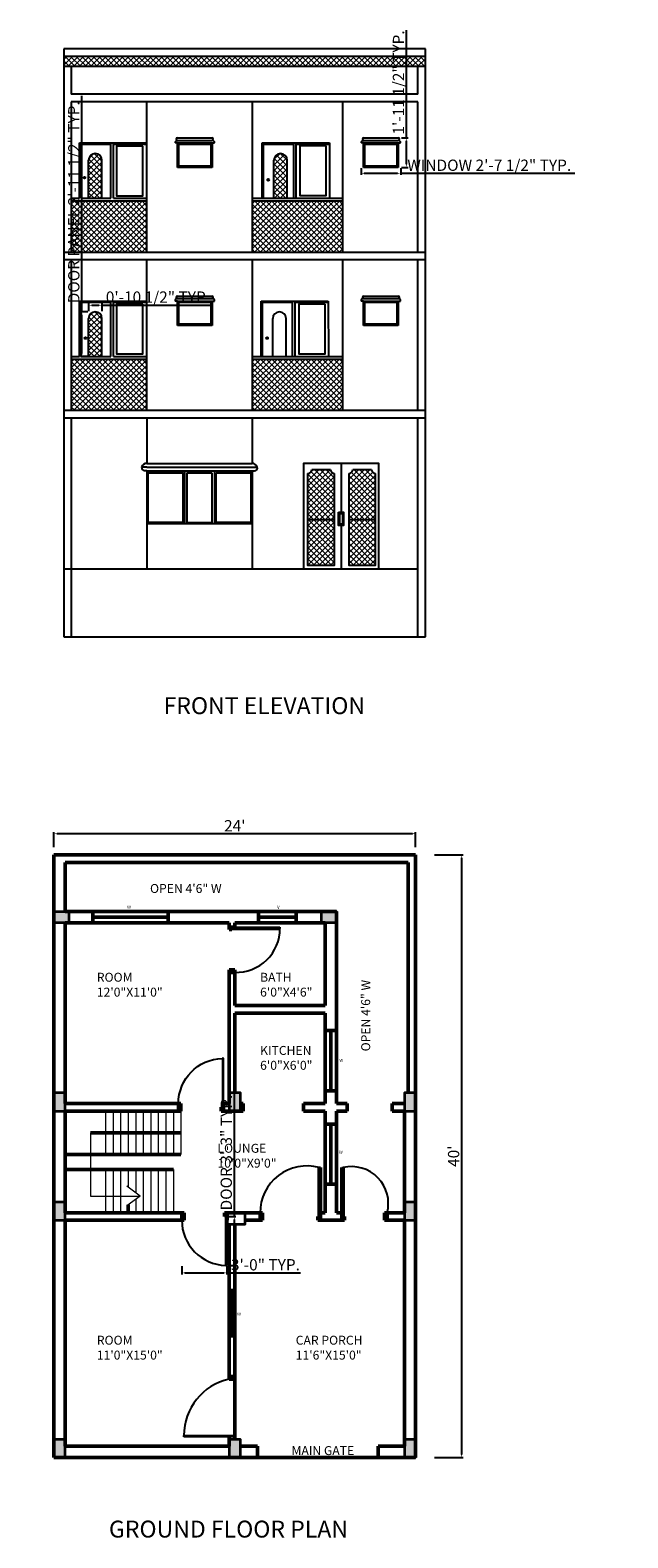
# Model space of a CAD drawing. Units: feet. Extents: x 1398 to 2768, y 682 to 1909.
# Tile 1 of 3: x 1398 to 1874, y 682 to 1883. Entities that reach past the tile are written whole.
import ezdxf

# ---------------------------------------------------------------- set-up
doc = ezdxf.new("R2010")
doc.units = ezdxf.units.FT
for name, color, linetype, lineweight in [('A-ANNO-DIMS', 2, 'Continuous', 18), ('A-ANNO-TEXT', 7, 'Continuous', 18), ('A-AREA-IDEN', 3, 'Continuous', 18), ('A-COLS', 7, 'Continuous', 35), ('A-DOOR', 4, 'Continuous', 25), ('A-ELEV', 7, 'Continuous', 25), ('A-ELEV-PATT', 8, 'Continuous', 13), ('A-FLOR-STRS', 3, 'Continuous', 18), ('A-WALL', 7, 'Continuous', 50), ('A-WALL-PATT', 8, 'Continuous', 13)]:
    doc.layers.add(name, color=color, linetype=linetype, lineweight=lineweight)
doc.styles.get("Standard").update_dxf_attribs({"font": 'arial.ttf'})
doc.dimstyles.new('ISO-25', dxfattribs={"dimtxt": 9, "dimasz": 2.5, "dimexe": 1.25, "dimexo": 0.625, "dimtad": 1, "dimdec": 1, "dimlunit": 3, "dimtxsty": 'Standard', "dimcen": 2.5, "dimadec": 0, "dimazin": 0, "dimtfac": 1, "dimtdec": 1, "dimtmove": 0, "dimatfit": 3, "dimfxl": 1, "dimarcsym": 0})
pattern_1 = [(45, (-71.1406, 0), (-2.245064, 2.245064), []), (135, (-71.1406, 0), (-2.245064, -2.245064), [])]

# ---------------------------------------------------------------- blocks, each defined once
blk = doc.blocks.new('*D1')
at = {"layer": 'A-ANNO-DIMS', "color": 0, "lineweight": -2, "transparency": 16777216}
for p, q in [((1416.8, 1232.1), (1416.8, 1244.2)), ((1702.3, 1242.9), (1419.3, 1242.9)), ((1704.8, 1232.1), (1704.8, 1244.2))]:
    blk.add_line(p, q, dxfattribs=at)
at = {"layer": 'A-ANNO-DIMS', "color": 0, "transparency": 16777216}
for points in [[(1419.3, 1243.4), (1419.3, 1242.5), (1416.8, 1242.9)], [(1702.3, 1243.4), (1702.3, 1242.5), (1704.8, 1242.9)]]:
    blk.add_solid(points, dxfattribs=at)
at = {"layer": 'Defpoints', "color": 0, "transparency": 16777216}
for p in [(1416.8, 1242.9), (1416.8, 1231.4), (1704.8, 1231.4)]:
    blk.add_point(p, dxfattribs=at)
at = {"layer": 'A-ANNO-DIMS', "color": 0, "transparency": 16777216, "insert": (1560.8, 1248.1), "char_height": 9, "attachment_point": 5}
blk.add_mtext("24'", dxfattribs=at)
blk = doc.blocks.new('*D2')
at = {"layer": 'A-ANNO-DIMS', "color": 0, "lineweight": -2, "transparency": 16777216}
for p, q in [((1719.8, 1226.1), (1742.7, 1226.1)), ((1741.4, 1223.6), (1741.4, 748.6)), ((1719.8, 746.1), (1742.7, 746.1))]:
    blk.add_line(p, q, dxfattribs=at)
at = {"layer": 'A-ANNO-DIMS', "color": 0, "transparency": 16777216}
for points in [[(1741, 1223.6), (1741.8, 1223.6), (1741.4, 1226.1)], [(1741, 748.6), (1741.8, 748.6), (1741.4, 746.1)]]:
    blk.add_solid(points, dxfattribs=at)
at = {"layer": 'Defpoints', "color": 0, "transparency": 16777216}
for p in [(1719.2, 1226.1), (1719.2, 746.1), (1741.4, 746.1)]:
    blk.add_point(p, dxfattribs=at)
at = {"layer": 'A-ANNO-DIMS', "color": 0, "transparency": 16777216, "insert": (1736.2, 986.1), "char_height": 9, "attachment_point": 5, "rotation": 90}
blk.add_mtext("40'", dxfattribs=at)
blk = doc.blocks.new('DOOR-PLAN-900')
for p, q in [((1553.6, 938.1), (1552.6, 938.1)), ((1553.6, 899.1), (1553.6, 938.1)), ((1554.6, 935.1), (1554.6, 899.1)), ((1554.6, 899.1), (1553.6, 899.1))]:
    blk.add_line(p, q)
blk.add_arc((1554.6, 935.1), 36, 180, 268.3861)
blk = doc.blocks.new('ELEV-WINDOW')
for p, q in [((2, 19.5), (0, 19.5)), ((2, 23.5), (29.5, 23.5)), ((2, 21.5), (29.5, 21.5)), ((2, 19.5), (29.5, 19.5)), ((2, 0), (2, 19.5)), ((29.5, 19.5), (29.5, 0)), ((29.5, 19.5), (31.5, 19.5)), ((29.5, 0), (2, 0))]:
    blk.add_line(p, q)
for centre, radius, start, end in [((2, 19.5), 2, 90, 180), ((2, 22.5), 1, 90, 270), ((29.5, 22.5), 1, 270, 90), ((29.5, 19.5), 2, 0, 90)]:
    blk.add_arc(centre, radius, start, end)
blk = doc.blocks.new('ELEV-DOOR')
for p, q in [((0, 0), (0, 30.3)), ((10.6, 0), (10.6, 30.3))]:
    blk.add_line(p, q)
blk.add_arc((5.3, 30.3), 5.3, 0, 180)
blk = doc.blocks.new('*D29')
at = {"layer": 'A-ANNO-DIMS', "color": 0, "lineweight": -2, "transparency": 16777216}
for p, q in [((1560.5, 938.1), (1560.5, 1037.5)), ((1555.2, 938.1), (1561.7, 938.1)), ((1560.5, 901.6), (1560.5, 935.6)), ((1555.2, 899.1), (1561.7, 899.1))]:
    blk.add_line(p, q, dxfattribs=at)
at = {"layer": 'A-ANNO-DIMS', "color": 0, "transparency": 16777216}
for points in [[(1560.1, 935.6), (1560.9, 935.6), (1560.5, 938.1)], [(1560.1, 901.6), (1560.9, 901.6), (1560.5, 899.1)]]:
    blk.add_solid(points, dxfattribs=at)
at = {"layer": 'Defpoints', "color": 0, "transparency": 16777216}
for p in [(1554.6, 938.1), (1560.5, 938.1), (1554.6, 899.1)]:
    blk.add_point(p, dxfattribs=at)
at = {"layer": 'A-ANNO-DIMS', "color": 0, "transparency": 16777216, "insert": (1555.2, 989), "char_height": 9, "attachment_point": 5, "rotation": 90}
blk.add_mtext('DOOR 3\'-3" TYP.', dxfattribs=at)
blk = doc.blocks.new('*D30')
at = {"layer": 'A-ANNO-DIMS', "color": 0, "lineweight": -2, "transparency": 16777216}
for p, q in [((1518.6, 898.5), (1518.6, 892)), ((1521.1, 893.2), (1552.1, 893.2)), ((1554.6, 898.5), (1554.6, 892)), ((1554.6, 893.2), (1613.2, 893.2))]:
    blk.add_line(p, q, dxfattribs=at)
at = {"layer": 'A-ANNO-DIMS', "color": 0, "transparency": 16777216}
for points in [[(1521.1, 893.6), (1521.1, 892.8), (1518.6, 893.2)], [(1552.1, 893.6), (1552.1, 892.8), (1554.6, 893.2)]]:
    blk.add_solid(points, dxfattribs=at)
at = {"layer": 'Defpoints', "color": 0, "transparency": 16777216}
for p in [(1518.6, 899.1), (1554.6, 899.1), (1554.6, 893.2)]:
    blk.add_point(p, dxfattribs=at)
at = {"layer": 'A-ANNO-DIMS', "color": 0, "transparency": 16777216, "insert": (1585.2, 898.5), "char_height": 9, "attachment_point": 5}
blk.add_mtext('3\'-0" TYP.', dxfattribs=at)
blk = doc.blocks.new('*D31')
at = {"layer": 'A-ANNO-DIMS', "color": 0, "lineweight": -2, "transparency": 16777216}
for p, q in [((1661.4, 1773), (1661.4, 1767.6)), ((1663.9, 1768.9), (1690.4, 1768.9)), ((1692.9, 1773), (1692.9, 1767.6)), ((1692.9, 1768.9), (1831.5, 1768.9))]:
    blk.add_line(p, q, dxfattribs=at)
at = {"layer": 'A-ANNO-DIMS', "color": 0, "transparency": 16777216}
for points in [[(1663.9, 1769.3), (1663.9, 1768.5), (1661.4, 1768.9)], [(1690.4, 1769.3), (1690.4, 1768.5), (1692.9, 1768.9)]]:
    blk.add_solid(points, dxfattribs=at)
at = {"layer": 'Defpoints', "color": 0, "transparency": 16777216}
for p in [(1661.4, 1773.6), (1692.9, 1773.6), (1692.9, 1768.9)]:
    blk.add_point(p, dxfattribs=at)
at = {"layer": 'A-ANNO-DIMS', "color": 0, "transparency": 16777216, "insert": (1763.4, 1774.1), "char_height": 9, "attachment_point": 5}
blk.add_mtext('WINDOW 2\'-7 1/2" TYP.', dxfattribs=at)
blk = doc.blocks.new('*D32')
at = {"layer": 'A-ANNO-DIMS', "color": 0, "lineweight": -2, "transparency": 16777216}
for p, q in [((1697.6, 1797.1), (1697.6, 1882.9)), ((1693.5, 1797.1), (1698.9, 1797.1)), ((1697.6, 1776.1), (1697.6, 1794.6)), ((1693.5, 1773.6), (1698.9, 1773.6))]:
    blk.add_line(p, q, dxfattribs=at)
at = {"layer": 'A-ANNO-DIMS', "color": 0, "transparency": 16777216}
for points in [[(1697.2, 1794.6), (1698, 1794.6), (1697.6, 1797.1)], [(1697.2, 1776.1), (1698, 1776.1), (1697.6, 1773.6)]]:
    blk.add_solid(points, dxfattribs=at)
at = {"layer": 'Defpoints', "color": 0, "transparency": 16777216}
for p in [(1692.9, 1797.1), (1697.6, 1797.1), (1692.9, 1773.6)]:
    blk.add_point(p, dxfattribs=at)
at = {"layer": 'A-ANNO-DIMS', "color": 0, "transparency": 16777216, "insert": (1692.3, 1841.2), "char_height": 9, "attachment_point": 5, "rotation": 90}
blk.add_mtext('1\'-11 1/2" TYP.', dxfattribs=at)
blk = doc.blocks.new('*D33')
at = {"layer": 'A-ANNO-DIMS', "color": 0, "lineweight": -2, "transparency": 16777216}
for p, q in [((1439.1, 1658.5), (1439.1, 1830.6)), ((1443.8, 1658.5), (1437.9, 1658.5)), ((1439.1, 1625.4), (1439.1, 1656)), ((1443.8, 1622.9), (1437.9, 1622.9))]:
    blk.add_line(p, q, dxfattribs=at)
at = {"layer": 'A-ANNO-DIMS', "color": 0, "transparency": 16777216}
for points in [[(1438.7, 1656), (1439.5, 1656), (1439.1, 1658.5)], [(1438.7, 1625.4), (1439.5, 1625.4), (1439.1, 1622.9)]]:
    blk.add_solid(points, dxfattribs=at)
at = {"layer": 'Defpoints', "color": 0, "transparency": 16777216}
for p in [(1439.1, 1658.5), (1444.5, 1658.5), (1444.5, 1622.9)]:
    blk.add_point(p, dxfattribs=at)
at = {"layer": 'A-ANNO-DIMS', "color": 0, "transparency": 16777216, "insert": (1433.8, 1745.8), "char_height": 9, "attachment_point": 5, "rotation": 90}
blk.add_mtext('DOOR PANEL 2\'-11 1/2" TYP.', dxfattribs=at)
blk = doc.blocks.new('*D34')
at = {"layer": 'A-ANNO-DIMS', "color": 0, "lineweight": -2, "transparency": 16777216}
for p, q in [((1444.5, 1659.1), (1444.5, 1665.1)), ((1447, 1663.8), (1452.6, 1663.8)), ((1455.1, 1659.1), (1455.1, 1665.1)), ((1455.1, 1663.8), (1541.6, 1663.8))]:
    blk.add_line(p, q, dxfattribs=at)
at = {"layer": 'A-ANNO-DIMS', "color": 0, "transparency": 16777216}
for points in [[(1447, 1664.2), (1447, 1663.4), (1444.5, 1663.8)], [(1452.6, 1664.2), (1452.6, 1663.4), (1455.1, 1663.8)]]:
    blk.add_solid(points, dxfattribs=at)
at = {"layer": 'Defpoints', "color": 0, "transparency": 16777216}
for p in [(1444.5, 1658.5), (1455.1, 1663.8), (1455.1, 1658.5)]:
    blk.add_point(p, dxfattribs=at)
at = {"layer": 'A-ANNO-DIMS', "color": 0, "transparency": 16777216, "insert": (1499.6, 1669.1), "char_height": 9, "attachment_point": 5}
blk.add_mtext('0\'-10 1/2" TYP.', dxfattribs=at)

msp = doc.modelspace()

# ---------------------------------------------------------------- hatches: boundary and pattern name
at = {"layer": 'A-ELEV-PATT'}
h = msp.add_hatch(dxfattribs=at)
h.set_pattern_fill('ANSI37', color=256, style=0)
h.set_pattern_definition(pattern_1)
h.paths.add_polyline_path([(1424.63, 1861.85), (1424.63, 1853.85), (1712.63, 1853.85), (1712.63, 1861.85)])
h = msp.add_hatch(dxfattribs=at)
h.set_pattern_fill('ANSI37', color=256, style=0)
h.set_pattern_definition(pattern_1)
h.paths.add_polyline_path([(1490.63, 1705.85), (1490.63, 1746.93), (1430.63, 1746.93), (1430.63, 1705.85)])
h.paths.add_polyline_path([(1574.63, 1746.93), (1574.63, 1705.85), (1646.63, 1705.85), (1646.63, 1746.93)])
h.paths.add_polyline_path([(1444.46, 1748.93), (1455.05, 1748.93), (1455.05, 1779.19, 1), (1444.46, 1779.19)])
h = msp.add_hatch(dxfattribs=at)
h.set_pattern_fill('ANSI37', color=256, style=0)
h.set_pattern_definition(pattern_1)
h.paths.add_polyline_path([(1591.97, 1748.93), (1602.56, 1748.93), (1602.56, 1779.19, 1), (1591.97, 1779.19)])
h = msp.add_hatch(dxfattribs=at)
h.set_pattern_fill('ANSI37', color=256, style=0)
h.set_pattern_definition(pattern_1)
h.paths.add_polyline_path([(1490.63, 1620.93), (1430.63, 1620.93), (1430.63, 1579.85), (1490.63, 1579.85)])
h.paths.add_polyline_path([(1646.63, 1620.93), (1574.63, 1620.93), (1574.63, 1579.85), (1646.63, 1579.85)])
h.paths.add_polyline_path([(1639.98, 1529.71, -0.3816711), (1636.94, 1533.08), (1622.1, 1533.08, -0.3824831), (1619.06, 1529.7), (1619.06, 1493.06), (1639.98, 1493.06)])
h.paths.add_polyline_path([(1672.7, 1529.71, -0.3816711), (1669.66, 1533.08), (1654.82, 1533.08, -0.3824831), (1651.78, 1529.7), (1651.78, 1493.06), (1672.7, 1493.06)])
h.paths.add_polyline_path([(1672.7, 1493.06), (1651.78, 1493.06), (1651.78, 1456.42), (1672.7, 1456.42)])
h.paths.add_polyline_path([(1639.98, 1493.06), (1619.06, 1493.06), (1619.06, 1456.42), (1639.98, 1456.42)])
h.paths.add_polyline_path([(1455.05, 1653.19, 1), (1444.46, 1653.19), (1444.46, 1622.93), (1455.05, 1622.93)])
at = {"layer": 'A-WALL-PATT'}
h = msp.add_hatch(dxfattribs=at)
h.set_pattern_fill('BRASS', color=256, scale=0.02, style=0)
h.paths.add_polyline_path([(1425.8, 949.48), (1416.8, 949.48), (1416.8, 935.08), (1425.8, 935.08)])
h.paths.add_polyline_path([(1416.8, 1022.08), (1425.8, 1022.08), (1425.8, 1036.48), (1416.8, 1036.48)])
h.paths.add_polyline_path([(1565.3, 1036.48), (1556.3, 1036.48), (1556.3, 1022.08), (1565.3, 1022.08)])
h.paths.add_polyline_path([(1704.8, 1022.08), (1704.8, 1036.48), (1695.8, 1036.48), (1695.8, 1022.08)])
h.paths.add_polyline_path([(1695.8, 935.08), (1704.8, 935.08), (1704.8, 949.48), (1695.8, 949.48)])
h.paths.add_polyline_path([(1704.8, 746.08), (1704.8, 760.48), (1695.8, 760.48), (1695.8, 746.08)])
h.paths.add_polyline_path([(1565.3, 746.08), (1565.3, 760.48), (1556.3, 760.48), (1556.3, 746.08)])
h.paths.add_polyline_path([(1425.8, 746.08), (1425.8, 760.48), (1416.8, 760.48), (1416.8, 746.08)])
h.paths.add_polyline_path([(1428.8, 1181.08), (1416.8, 1181.08), (1416.8, 1172.09), (1428.8, 1172.09)])
h.paths.add_polyline_path([(1629.8, 1181.08), (1629.8, 1172.09), (1641.8, 1172.09), (1641.8, 1181.08)])
h.paths.add_polyline_path([(1937.94, 1022.08), (1946.94, 1022.08), (1946.94, 1036.48), (1937.94, 1036.48)])
h.paths.add_polyline_path([(1946.94, 949.48), (1937.94, 949.48), (1937.94, 935.08), (1946.94, 935.08)])
h.paths.add_polyline_path([(1946.94, 760.48), (1937.94, 760.48), (1937.94, 746.08), (1946.94, 746.08)])
h.paths.add_polyline_path([(2077.44, 746.08), (2086.44, 746.08), (2086.44, 760.48), (2077.44, 760.48)])
h.paths.add_polyline_path([(2070.54, 941.08), (2084.94, 941.08), (2084.94, 950.08), (2070.54, 950.08)])
h.paths.add_polyline_path([(2086.44, 1036.48), (2077.44, 1036.48), (2077.44, 1022.08), (2086.44, 1022.08)])
h.paths.add_polyline_path([(2162.94, 1172.09), (2162.94, 1181.08), (2150.94, 1181.08), (2150.94, 1172.09)])
h.paths.add_polyline_path([(1949.94, 1172.09), (1949.94, 1181.08), (1937.94, 1181.08), (1937.94, 1172.09)])
h.paths.add_polyline_path([(2216.94, 1022.08), (2225.94, 1022.08), (2225.94, 1036.48), (2216.94, 1036.48)])
h.paths.add_polyline_path([(2225.94, 935.08), (2225.94, 949.48), (2216.94, 949.48), (2216.94, 935.08)])
h.paths.add_polyline_path([(2216.94, 746.08), (2225.94, 746.08), (2225.94, 760.48), (2216.94, 760.48)])
h.paths.add_polyline_path([(2489.29, 760.48), (2480.29, 760.48), (2480.29, 746.08), (2489.29, 746.08)])
h.paths.add_polyline_path([(2628.79, 746.08), (2628.79, 760.48), (2619.79, 760.48), (2619.79, 746.08)])
h.paths.add_polyline_path([(2768.29, 760.48), (2759.29, 760.48), (2759.29, 746.08), (2768.29, 746.08)])
h.paths.add_polyline_path([(2768.29, 949.48), (2759.29, 949.48), (2759.29, 935.08), (2768.29, 935.08)])
h.paths.add_polyline_path([(2619.79, 926.68), (2628.79, 926.68), (2628.79, 941.08), (2619.79, 941.08)])
h.paths.add_polyline_path([(2489.29, 949.48), (2480.29, 949.48), (2480.29, 935.08), (2489.29, 935.08)])
h.paths.add_polyline_path([(2480.29, 1022.08), (2489.29, 1022.08), (2489.29, 1036.48), (2480.29, 1036.48)])
h.paths.add_polyline_path([(2628.79, 1036.48), (2619.79, 1036.48), (2619.79, 1022.08), (2628.79, 1022.08)])
h.paths.add_polyline_path([(2759.29, 1022.08), (2768.29, 1022.08), (2768.29, 1036.48), (2759.29, 1036.48)])
h.paths.add_polyline_path([(2693.29, 1172.09), (2705.29, 1172.09), (2705.29, 1181.08), (2693.29, 1181.08)])
h.paths.add_polyline_path([(2492.29, 1181.08), (2480.29, 1181.08), (2480.29, 1172.09), (2492.29, 1172.09)])
h = msp.add_hatch(dxfattribs=at)
h.set_pattern_fill('AR-B816', color=256, style=0)
h.paths.add_polyline_path([(1569.02, 932.08), (1569.02, 941.08), (1554.62, 941.08), (1554.62, 932.08)])

# ---------------------------------------------------------------- linework, layer by layer
at = {"layer": 'A-COLS'}
for points in [[(1416.8, 1181.08), (1428.8, 1181.08), (1428.8, 1172.09), (1416.8, 1172.09)], [(1629.8, 1181.08), (1641.8, 1181.08), (1641.8, 1172.09), (1629.8, 1172.09)], [(1416.8, 1022.08), (1425.8, 1022.08), (1425.8, 1036.48), (1416.8, 1036.48)], [(1556.3, 1022.08), (1565.3, 1022.08), (1565.3, 1036.48), (1556.3, 1036.48)], [(1695.8, 1022.08), (1704.8, 1022.08), (1704.8, 1036.48), (1695.8, 1036.48)], [(1416.8, 935.08), (1425.8, 935.08), (1425.8, 949.48), (1416.8, 949.48)], [(1695.8, 935.08), (1704.8, 935.08), (1704.8, 949.48), (1695.8, 949.48)], [(1554.62, 941.08), (1554.62, 932.08), (1569.02, 932.08), (1569.02, 941.08)], [(1416.8, 746.08), (1425.8, 746.08), (1425.8, 760.48), (1416.8, 760.48)], [(1556.3, 746.08), (1565.3, 746.08), (1565.3, 760.48), (1556.3, 760.48)], [(1695.8, 746.08), (1704.8, 746.08), (1704.8, 760.48), (1695.8, 760.48)]]:
    msp.add_lwpolyline(points, close=True, dxfattribs=at)
at = {"layer": 'A-DOOR'}
for p, q in [((1560.8, 1168.53), (1596.8, 1168.53)), ((1596.8, 1168.53), (1596.8, 1167.53)), ((1628.92, 977.08), (1627.92, 977.08)), ((1646.05, 977.08), (1647.05, 977.08)), ((1520.3, 762.65), (1520.3, 763.65)), ((1520.3, 763.65), (1560.8, 763.65)), ((1556.3, 762.65), (1520.3, 762.65)), ((1560.8, 762.65), (1556.3, 762.65))]:
    msp.add_line(p, q, dxfattribs=at)
for centre, radius, start, end in [((1561.79, 1167.53), 35.01, 268.38614, 360), ((1618.2, 941.08), 37.29, 74.90116, 180), ((1653.79, 948.62), 29.25, 345.05973, 103.32641), ((1566.43, 763.65), 46.13, 102.68038, 180)]:
    msp.add_arc(centre, radius, start, end, dxfattribs=at)
at = {"layer": 'A-ELEV'}
for p, q in [((1712.63, 1867.85), (1424.63, 1867.85)), ((1424.63, 1867.85), (1424.63, 1399.85)), ((1712.63, 1861.85), (1424.63, 1861.85)), ((1712.63, 1831.85), (1712.63, 1867.85)), ((1712.63, 1853.85), (1424.63, 1853.85)), ((1430.63, 1853.85), (1430.63, 1831.85)), ((1706.63, 1831.85), (1706.63, 1853.85)), ((1706.63, 1831.85), (1430.63, 1831.85)), ((1706.63, 1825.85), (1430.63, 1825.85)), ((1430.63, 1825.85), (1430.63, 1705.85)), ((1430.63, 1825.85), (1430.63, 1705.85)), ((1490.63, 1825.85), (1490.63, 1705.85)), ((1574.63, 1825.85), (1574.63, 1705.85)), ((1646.63, 1825.85), (1646.63, 1705.85)), ((1706.63, 1705.85), (1706.63, 1825.85)), ((1712.63, 1399.85), (1712.63, 1831.85)), ((1437.19, 1748.93), (1437.19, 1793.13)), ((1437.19, 1793.13), (1490.63, 1793.13)), ((1438.19, 1748.93), (1438.19, 1792.13)), ((1438.19, 1792.13), (1462.19, 1792.13)), ((1462.19, 1748.93), (1462.19, 1792.13)), ((1464.19, 1748.93), (1464.19, 1792.13)), ((1464.19, 1792.13), (1490.63, 1792.13)), ((1582.7, 1748.93), (1582.7, 1793.13)), ((1582.7, 1793.13), (1636.14, 1793.13)), ((1583.7, 1748.93), (1583.7, 1792.13)), ((1583.7, 1792.13), (1607.7, 1792.13)), ((1607.7, 1748.93), (1607.7, 1792.13)), ((1609.7, 1748.93), (1609.7, 1792.13)), ((1609.7, 1792.13), (1636.14, 1792.13)), ((1636.14, 1793.13), (1636.28, 1748.93)), ((1430.63, 1748.93), (1437.19, 1748.93)), ((1430.63, 1746.93), (1490.63, 1746.93)), ((1438.19, 1748.93), (1462.19, 1748.93)), ((1464.19, 1748.93), (1490.63, 1748.93)), ((1574.63, 1748.93), (1646.63, 1748.93)), ((1574.63, 1746.93), (1646.63, 1746.93)), ((1610.63, 1705.85), (1424.63, 1705.85)), ((1712.63, 1705.85), (1424.63, 1705.85)), ((1712.63, 1705.85), (1610.63, 1705.85)), ((1610.63, 1699.85), (1424.63, 1699.85)), ((1430.63, 1699.85), (1430.63, 1579.85)), ((1490.63, 1699.85), (1490.63, 1579.85)), ((1574.63, 1699.85), (1574.63, 1579.85)), ((1712.63, 1699.85), (1610.63, 1699.85)), ((1646.63, 1699.85), (1646.63, 1579.85)), ((1706.63, 1579.85), (1706.63, 1699.85)), ((1437.19, 1622.93), (1437.19, 1667.13)), ((1437.19, 1667.13), (1490.63, 1667.13)), ((1438.19, 1622.93), (1438.19, 1666.13)), ((1438.19, 1666.13), (1462.19, 1666.13)), ((1462.19, 1622.93), (1462.19, 1666.13)), ((1464.19, 1622.93), (1464.19, 1666.13)), ((1464.19, 1666.13), (1490.63, 1666.13)), ((1581.8, 1622.93), (1581.8, 1667.13)), ((1581.8, 1667.13), (1635.25, 1667.13)), ((1582.8, 1622.93), (1582.8, 1666.13)), ((1582.8, 1666.13), (1606.8, 1666.13)), ((1606.8, 1622.93), (1606.8, 1666.13)), ((1608.8, 1622.93), (1608.8, 1666.13)), ((1608.8, 1666.13), (1635.25, 1666.13)), ((1635.25, 1667.13), (1635.38, 1622.93)), ((1430.63, 1622.93), (1437.19, 1622.93)), ((1430.63, 1620.93), (1490.63, 1620.93)), ((1438.19, 1622.93), (1462.19, 1622.93)), ((1464.19, 1622.93), (1490.63, 1622.93)), ((1574.63, 1622.93), (1646.63, 1622.93)), ((1574.63, 1620.93), (1646.63, 1620.93)), ((1712.63, 1579.85), (1424.63, 1579.85)), ((1712.63, 1573.85), (1424.63, 1573.85)), ((1430.63, 1573.85), (1430.63, 1399.85)), ((1490.65, 1573.85), (1490.65, 1537.85)), ((1574.63, 1573.85), (1574.63, 1537.85)), ((1706.63, 1399.85), (1706.63, 1573.85)), ((1490.65, 1537.85), (1574.63, 1537.85)), ((1645.53, 1537.85), (1645.53, 1499.05)), ((1490.65, 1534.85), (1486.65, 1534.85)), ((1490.65, 1531.85), (1488.65, 1531.85)), ((1490.65, 1534.85), (1574.63, 1534.85)), ((1490.65, 1531.85), (1574.63, 1531.85)), ((1490.65, 1531.85), (1490.65, 1453.85)), ((1520.65, 1531.85), (1520.65, 1489.85)), ((1522.65, 1530.23), (1522.65, 1490.86)), ((1522.65, 1530.23), (1542.63, 1530.23)), ((1542.63, 1530.23), (1542.63, 1490.86)), ((1544.63, 1531.85), (1544.63, 1489.85)), ((1574.63, 1534.85), (1578.63, 1534.85)), ((1574.63, 1531.85), (1576.63, 1531.85)), ((1574.63, 1531.85), (1574.63, 1489.85)), ((1574.63, 1531.85), (1574.63, 1453.85)), ((1490.65, 1489.85), (1574.63, 1489.85)), ((1522.65, 1490.86), (1542.63, 1490.86)), ((1619.06, 1493.06), (1639.98, 1493.06)), ((1651.78, 1493.06), (1672.7, 1493.06)), ((1645.53, 1488.39), (1645.53, 1453.85)), ((1424.63, 1453.85), (1706.63, 1453.85)), ((1424.63, 1399.85), (1712.63, 1399.85))]:
    msp.add_line(p, q, dxfattribs=at)
for points in [[(1487.72, 1790.52), (1466.62, 1790.52), (1466.62, 1751.04), (1487.72, 1751.04)], [(1516.22, 1792.13), (1541.75, 1792.13), (1541.75, 1774.6), (1516.22, 1774.6)], [(1633.69, 1790.62), (1612.59, 1790.62), (1612.59, 1751.14), (1633.69, 1751.14)], [(1664.36, 1792.13), (1689.89, 1792.13), (1689.89, 1774.6), (1664.36, 1774.6)], [(1487.72, 1664.62), (1466.62, 1664.62), (1466.62, 1625.14), (1487.72, 1625.14)], [(1516.22, 1666.13), (1541.75, 1666.13), (1541.75, 1648.6), (1516.22, 1648.6)], [(1632.79, 1664.62), (1611.7, 1664.62), (1611.7, 1625.14), (1632.79, 1625.14)], [(1664.36, 1666.13), (1689.89, 1666.13), (1689.89, 1648.6), (1664.36, 1648.6)], [(1615.53, 1453.85), (1675.53, 1453.85), (1675.53, 1537.85), (1615.53, 1537.85)], [(1491.84, 1530.23), (1519.32, 1530.23), (1519.32, 1490.86), (1491.84, 1490.86)], [(1545.98, 1530.23), (1573.45, 1530.23), (1573.45, 1490.86), (1545.98, 1490.86)], [(1643.44, 1499.05), (1647.49, 1499.05), (1647.49, 1488.39), (1643.44, 1488.39)], [(1644.44, 1498.05), (1646.49, 1498.05), (1646.49, 1489.39), (1644.44, 1489.39)]]:
    msp.add_lwpolyline(points, close=True, dxfattribs=at)
for points in [[(1639.98, 1529.71), (1639.98, 1456.42), (1619.06, 1456.42), (1619.06, 1529.7)], [(1622.1, 1533.08), (1636.94, 1533.08)], [(1672.7, 1529.71), (1672.7, 1456.42), (1651.78, 1456.42), (1651.78, 1529.7)], [(1654.82, 1533.08), (1669.66, 1533.08)]]:
    msp.add_lwpolyline(points, dxfattribs=at)
for centre in [(1441.2, 1765.37), (1587.45, 1763.65), (1441.94, 1637.65), (1586.55, 1637.65)]:
    msp.add_circle(centre, 0.696, dxfattribs=at)
for centre, radius, start, end in [((1490.65, 1533.68), 4.17, 90, 163.7398), ((1574.63, 1533.68), 4.17, 16.2602, 90), ((1489.9, 1534.85), 3.25, 180, 247.38014), ((1576.63, 1534.01), 2.17, 270, 22.61986), ((1618.69, 1533.08), 3.41, 276.27597, 360), ((1640.35, 1533.09), 3.41, 180, 263.72403), ((1651.41, 1533.08), 3.41, 276.27597, 360), ((1673.07, 1533.09), 3.41, 180, 263.72403)]:
    msp.add_arc(centre, radius, start, end, dxfattribs=at)
at = {"layer": 'A-FLOR-STRS'}
for p, q in [((1457.91, 1022.08), (1457.91, 987.58)), ((1463.91, 1022.08), (1463.91, 987.58)), ((1469.91, 1022.08), (1469.91, 987.58)), ((1475.91, 1022.08), (1475.91, 987.58)), ((1481.91, 1022.08), (1481.91, 987.58)), ((1487.91, 1022.08), (1487.91, 987.58)), ((1493.91, 1022.08), (1493.91, 987.58)), ((1499.91, 1022.08), (1499.91, 987.58)), ((1505.91, 1022.08), (1505.91, 987.58)), ((1511.91, 1022.08), (1511.91, 987.58)), ((1517.91, 1022.08), (1517.91, 987.58)), ((1446, 1004.83), (1446, 954.35)), ((1457.91, 975.58), (1457.91, 941.08)), ((1463.91, 975.58), (1463.91, 941.08)), ((1469.91, 975.58), (1469.91, 941.08)), ((1475.91, 975.58), (1475.91, 961.37)), ((1481.91, 975.58), (1481.91, 956.91)), ((1487.91, 975.58), (1487.91, 941.08)), ((1493.91, 975.58), (1493.91, 941.08)), ((1499.91, 975.58), (1499.91, 941.08)), ((1505.91, 975.58), (1505.91, 941.08)), ((1511.91, 975.58), (1511.91, 941.08)), ((1485.36, 954.35), (1474.89, 962.13)), ((1446, 954.35), (1485.36, 954.35)), ((1485.36, 954.35), (1474.89, 946.57)), ((1481.91, 951.79), (1481.91, 941.08))]:
    msp.add_line(p, q, dxfattribs=at)
at = {"layer": 'A-WALL'}
for p, q in [((1704.8, 1226.08), (1416.8, 1226.08)), ((1416.8, 1226.08), (1416.8, 746.08)), ((1704.8, 746.08), (1704.8, 1226.08)), ((1425.8, 1220.08), (1425.8, 1181.08)), ((1698.8, 1220.08), (1425.8, 1220.08)), ((1698.8, 1036.48), (1698.8, 1220.08)), ((1641.8, 1181.08), (1425.8, 1181.08)), ((1447.68, 1181.08), (1447.68, 1172.08)), ((1507.68, 1181.08), (1507.68, 1172.08)), ((1579.68, 1181.08), (1579.68, 1172.08)), ((1609.68, 1181.08), (1609.68, 1172.08)), ((1641.8, 1028.08), (1641.8, 1181.08)), ((1425.8, 1172.08), (1425.8, 1028.08)), ((1556.3, 1172.08), (1425.8, 1172.08)), ((1447.68, 1176.58), (1507.68, 1176.58)), ((1556.3, 1166.55), (1556.3, 1172.08)), ((1560.8, 1168.53), (1556.3, 1168.53)), ((1558.55, 1166.55), (1556.3, 1166.55)), ((1596.8, 1167.53), (1558.55, 1167.53)), ((1558.55, 1167.53), (1558.55, 1166.55)), ((1632.8, 1172.08), (1560.8, 1172.08)), ((1560.8, 1167.53), (1560.8, 1172.08)), ((1579.68, 1176.58), (1609.68, 1176.58)), ((1632.8, 1106.08), (1632.8, 1172.08)), ((1556.3, 1028.08), (1556.3, 1134.53)), ((1560.8, 1134.53), (1556.3, 1134.53)), ((1560.8, 1132.53), (1556.3, 1132.53)), ((1560.8, 1106.08), (1560.8, 1134.53)), ((1560.8, 1106.08), (1632.8, 1106.08)), ((1560.8, 1036.48), (1560.8, 1100.08)), ((1560.8, 1100.08), (1632.8, 1100.08)), ((1632.8, 1028.08), (1632.8, 1100.08)), ((1632.8, 1086.15), (1641.8, 1086.15)), ((1637.3, 1086.15), (1637.3, 1038.15)), ((1632.8, 1038.15), (1641.8, 1038.15)), ((1517.91, 1028.08), (1425.8, 1028.08)), ((1425.8, 1022.08), (1425.8, 941.08)), ((1517.91, 1022.08), (1425.8, 1022.08)), ((1515.91, 1028.08), (1515.91, 1022.08)), ((1517.91, 1028.08), (1517.91, 1022.08)), ((1549.91, 1025.08), (1549.91, 1022.08)), ((1556.3, 1022.08), (1549.91, 1022.08)), ((1556.3, 1028.08), (1551.91, 1028.08)), ((1551.91, 1028.08), (1551.91, 1022.08)), ((1556.3, 1022.08), (1567.51, 1022.08)), ((1565.3, 1028.08), (1567.51, 1028.08)), ((1567.51, 1028.08), (1567.51, 1022.08)), ((1615.51, 1028.08), (1615.51, 1022.08)), ((1615.51, 1028.08), (1632.8, 1028.08)), ((1615.51, 1022.08), (1632.8, 1022.08)), ((1632.8, 941.08), (1632.8, 1022.08)), ((1641.8, 1028.08), (1650.24, 1028.08)), ((1641.8, 941.08), (1641.8, 1022.08)), ((1641.8, 1022.08), (1650.24, 1022.08)), ((1650.24, 1028.08), (1650.24, 1022.08)), ((1686.24, 1028.08), (1686.24, 1022.08)), ((1686.24, 1028.08), (1695.8, 1028.08)), ((1686.24, 1022.08), (1695.8, 1022.08)), ((1695.8, 941.08), (1695.8, 1022.08)), ((1632.8, 1011.76), (1641.8, 1011.76)), ((1637.3, 1011.76), (1637.3, 963.76)), ((1517.91, 1004.83), (1446, 1004.83)), ((1517.91, 987.58), (1425.8, 987.58)), ((1511.91, 975.58), (1425.8, 975.58)), ((1627.92, 977.08), (1627.92, 938.08)), ((1628.92, 941.08), (1628.92, 977.08)), ((1646.05, 941.08), (1646.05, 977.08)), ((1647.05, 977.08), (1647.05, 938.08)), ((1632.8, 963.76), (1641.8, 963.76)), ((1425.8, 941.08), (1520.62, 941.08)), ((1475.91, 947.33), (1475.91, 941.08)), ((1518.62, 941.08), (1518.62, 935.08)), ((1520.62, 941.08), (1520.62, 935.08)), ((1552.62, 938.08), (1552.62, 941.08)), ((1552.62, 941.08), (1582.92, 941.08)), ((1554.62, 941.08), (1554.62, 935.08)), ((1580.92, 941.08), (1580.92, 935.08)), ((1582.92, 941.08), (1582.92, 935.08)), ((1627.92, 938.08), (1626.92, 938.08)), ((1626.92, 938.08), (1626.92, 935.08)), ((1627.92, 941.08), (1632.8, 941.08)), ((1628.92, 941.08), (1628.92, 935.08)), ((1641.8, 941.08), (1647.05, 941.08)), ((1646.05, 941.08), (1646.05, 935.08)), ((1647.05, 938.08), (1648.03, 938.08)), ((1648.03, 938.08), (1648.03, 935.08)), ((1680.05, 941.08), (1680.05, 935.08)), ((1680.05, 941.08), (1695.8, 941.08)), ((1682.05, 941.08), (1682.05, 935.08)), ((1425.8, 935.08), (1520.62, 935.08)), ((1425.8, 935.08), (1425.8, 755.08)), ((1556.3, 808.65), (1556.3, 932.08)), ((1560.8, 760.48), (1560.8, 932.08)), ((1569.02, 935.08), (1582.92, 935.08)), ((1626.92, 935.08), (1648.03, 935.08)), ((1680.05, 935.08), (1695.8, 935.08)), ((1695.8, 755.08), (1695.8, 935.08)), ((1560.8, 879.04), (1556.3, 879.04)), ((1558.55, 879.04), (1558.55, 843.04)), ((1560.8, 843.04), (1556.3, 843.04)), ((1560.8, 810.65), (1556.3, 810.65)), ((1560.8, 808.65), (1556.3, 808.65)), ((1556.3, 755.08), (1556.3, 762.65)), ((1416.8, 746.08), (1578.91, 746.08)), ((1425.8, 755.08), (1556.3, 755.08)), ((1565.3, 755.08), (1578.91, 755.08)), ((1578.91, 755.08), (1578.91, 746.08)), ((1578.91, 746.08), (1674.91, 746.08)), ((1674.91, 755.08), (1674.91, 746.08)), ((1674.91, 755.08), (1695.8, 755.08)), ((1674.91, 746.08), (1704.8, 746.08))]:
    msp.add_line(p, q, dxfattribs=at)

# ---------------------------------------------------------------- block references
at = {"layer": 'A-DOOR', "extrusion": (0, 0, -1), "zscale": -1, "rotation": 180}
msp.add_blockref('DOOR-PLAN-900', (2.71, 1963.16), dxfattribs=at)
at = {"layer": 'A-DOOR'}
msp.add_blockref('DOOR-PLAN-900', (0, 0), dxfattribs=at)
at = {"layer": 'A-ELEV'}
for name, p in [('ELEV-WINDOW', (1513.22, 1773.6)), ('ELEV-WINDOW', (1661.36, 1773.6)), ('ELEV-DOOR', (1444.46, 1748.93)), ('ELEV-DOOR', (1591.97, 1748.93)), ('ELEV-WINDOW', (1513.22, 1647.6)), ('ELEV-WINDOW', (1661.36, 1647.6)), ('ELEV-DOOR', (1444.46, 1622.93)), ('ELEV-DOOR', (1591.07, 1622.93))]:
    msp.add_blockref(name, p, dxfattribs=at)

# ---------------------------------------------------------------- texts
at = {"layer": 'A-ANNO-TEXT', "attachment_point": 1}
for s, width, gutter_width, insert, char_height in [('FRONT ELEVATION', 449.1316, 67.3, (1504.11, 1351.62), 13.4591), ('W', 29.3663, 12.5, (1475.09, 1185.75), 2.5), ('V', 29.3663, 12.5, (1594.46, 1185.59), 2.5), ('W', 29.3663, 12.5, (1644.1, 1063.54), 2.5), ('W', 29.3663, 12.5, (1643.75, 990.65), 2.5), ('W', 29.3663, 12.5, (1562.67, 861.63), 2.5), ('GROUND FLOOR PLAN ', 449.1316, 67.3, (1460.6, 695.89), 13.4591)]:
    msp.add_mtext_dynamic_manual_height_columns(s, width=width, gutter_width=gutter_width, heights=[0], dxfattribs=dict(at, insert=insert, char_height=char_height))
at = {"layer": 'A-AREA-IDEN', "attachment_point": 1}
for s, insert, char_height in [('OPEN 4\'6" W', (1493.33, 1202.86), 7.1088), ('ROOM \\P12\'0"X11\'0"', (1450.95, 1132.18), 7.1088), ('BATH\\P6\'0"X4\'6"', (1580.95, 1132.18), 7.109), ('KITCHEN\\P6\'0"X6\'0"', (1580.95, 1073.9), 7.109), ('LOUNGE  \\P10\'0"X9\'0"', (1547, 995.98), 7.109), ('ROOM \\P11\'0"X15\'0"', (1450.95, 843.13), 7.1088), ('CAR PORCH\\P11\'6"X15\'0"', (1609.33, 843.13), 7.1088), ('MAIN GATE', (1605.99, 755.22), 7.109)]:
    msp.add_mtext_dynamic_manual_height_columns(s, width=237.2218, gutter_width=35.54, heights=[0], dxfattribs=dict(at, insert=insert, char_height=char_height))
at = {"layer": 'A-AREA-IDEN', "insert": (1661.49, 1069.6), "char_height": 7.1088, "attachment_point": 1, "rotation": 90}
msp.add_mtext_dynamic_manual_height_columns('OPEN 4\'6" W', width=237.2218, gutter_width=35.54, heights=[0], dxfattribs=at)

# ---------------------------------------------------------------- dimensions: what is measured, and where the dimension line sits
at = {"layer": 'A-ANNO-DIMS'}
for base, p1, p2, text, picture, middle in [((1697.62, 1797.13), (1692.89, 1773.6), (1692.89, 1797.13), '<> TYP.', '*D32', (1692.34, 1841.24)), ((1439.12, 1658.49), (1444.46, 1622.93), (1444.46, 1658.49), 'DOOR PANEL <> TYP.', '*D33', (1433.84, 1745.77)), ((1560.47, 938.08), (1554.62, 899.08), (1554.62, 938.08), 'DOOR <> TYP.', '*D29', (1555.18, 989.02))]:
    dim = msp.add_linear_dim(base=base, p1=p1, p2=p2, angle=90, text=text, dimstyle='ISO-25', override={"dimdec": 1, "dimrnd": 0, "dimzin": 1, "dimlunit": 4, "dimfrac": 2}, dxfattribs=at)
    dim.commit()
    dim.dimension.update_dxf_attribs({"geometry": picture, "text_midpoint": middle})
for base, p1, p2, text, picture, middle in [((1692.89, 1768.87), (1661.36, 1773.6), (1692.89, 1773.6), 'WINDOW <> TYP.', '*D31', (1763.44, 1774.15)), ((1455.05, 1663.83), (1444.46, 1658.49), (1455.05, 1658.49), '<> TYP.', '*D34', (1499.59, 1669.1)), ((1554.62, 893.23), (1518.62, 899.08), (1554.62, 899.08), '<> TYP.', '*D30', (1585.17, 898.46))]:
    dim = msp.add_linear_dim(base=base, p1=p1, p2=p2, text=text, dimstyle='ISO-25', override={"dimdec": 1, "dimrnd": 0, "dimzin": 1, "dimlunit": 4, "dimfrac": 2}, dxfattribs=at)
    dim.commit()
    dim.dimension.update_dxf_attribs({"geometry": picture, "text_midpoint": middle})
dim = msp.add_linear_dim(base=(1416.8, 1242.95), p1=(1704.8, 1231.43), p2=(1416.8, 1231.43), dimstyle='ISO-25', override={"dimclrd": 0, "dimclre": 0, "dimclrt": 0}, dxfattribs=at)
dim.commit()
dim.dimension.update_dxf_attribs({"geometry": '*D1', "text_midpoint": (1560.8, 1248.09)})
dim = msp.add_linear_dim(base=(1741.43, 746.08), p1=(1719.16, 1226.08), p2=(1719.16, 746.08), angle=90, dimstyle='ISO-25', override={"dimclrd": 0, "dimclre": 0, "dimclrt": 0}, dxfattribs=at)
dim.commit()
dim.dimension.update_dxf_attribs({"geometry": '*D2', "text_midpoint": (1736.21, 986.08)})

doc.saveas('drawing.dxf')
